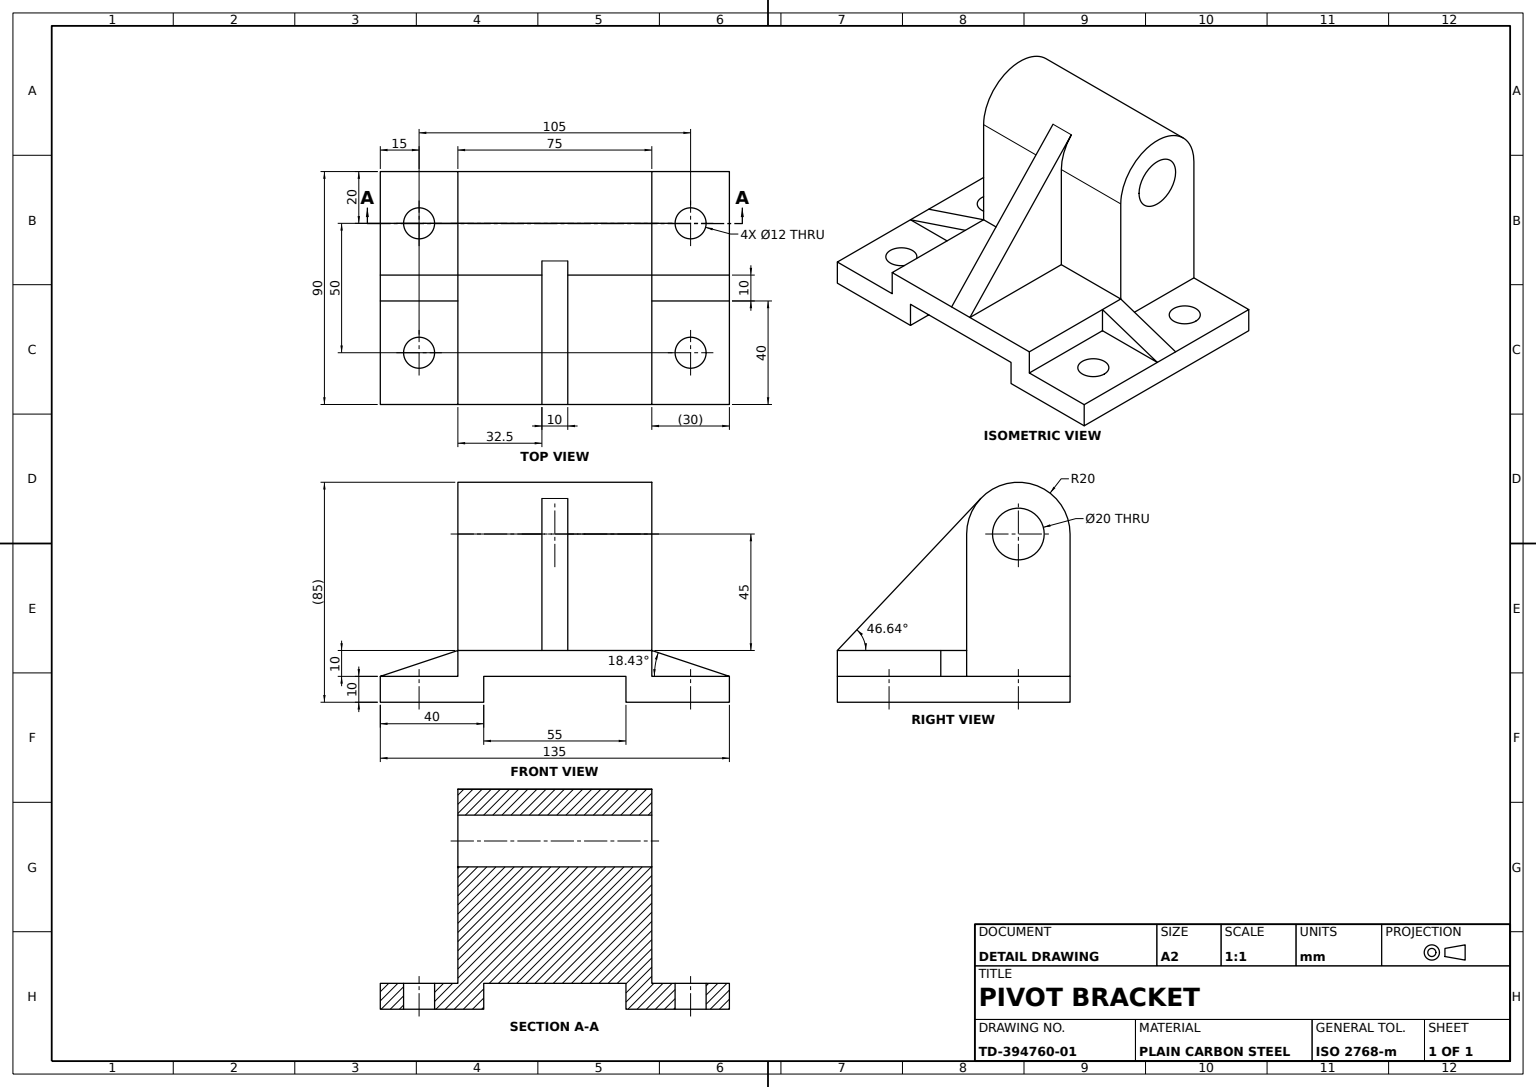
SolidWorks part; units mm, degrees
material "Plain Carbon Steel"
ref_plane "Front Plane" through (0, 0, 0) normal (0, 0, 1) x (1, 0, 0)
ref_plane "Top Plane" through (0, 0, 0) normal (0, 1, 0) x (1, 0, 0)
ref_plane "Right Plane" through (0, 0, 0) normal (1, 0, 0) x (0, 0, -1)
sketch "Base Plate Profile" plane through (0, 0, 0) normal (0, 0, 1) x (1, 0, 0)
  line L0 (-67.5, 0) -> (-27.5, 0)
  line L1 (-27.5, 0) -> (-27.5, 10)
  line L2 (-27.5, 10) -> (27.5, 10)
  line L3 (27.5, 10) -> (27.5, 0)
  line L4 (27.5, 0) -> (67.5, 0)
  line L5 (67.5, 0) -> (67.5, 10)
  line L7 (-67.5, 10) -> (-67.5, 0)
  line L8 (67.5, 10) -> (37.5, 10)
  line L9 (37.5, 10) -> (37.5, 20)
  line L10 (37.5, 20) -> (-37.5, 20)
  line L11 (-37.5, 20) -> (-37.5, 10)
  line L12 (-37.5, 10) -> (-67.5, 10)
  line L13 (0, 0) -> (0, 63.9926) construction
  line L14 (0, 0) -> (111.5972, 0) construction
  dimension "D1" = 55
  dimension "D2" = 135
  dimension "D3" = 75
  dimension "D4" = 10
  dimension "D5" = 10
  dimension "D6" = 10
  dimension "D7" = 10
extrude "Base Plate" add sketch "Base Plate Profile" along normal mid plane 90 contours L2 L3 L4 L5 L8 L9 L10 L11 L12 L7 L0 L1
sketch "Mounting Holes Sketch" plane through (0, 10, 0) normal (0, 1, 0) x (1, 0, 0)
  line L0 (0, 0) -> (0, -31.826) construction
  line L1 (67.5, -45) -> (37.5, -45) construction
  line L2 (67.5, 45) -> (37.5, 45) construction
  line L3 (37.5, -45) -> (37.5, 45) construction
  line L4 (37.5, -45) -> (37.5, 45) construction
  circle A0 centre (52.5, -25) radius 6
  circle A1 centre (52.5, 25) radius 6
  circle A2 centre (-52.5, 25) radius 6
  circle A3 centre (-52.5, -25) radius 6
  dimension "D1" = 12
  dimension "D2" = 12
  dimension "D3" = 20
  dimension "D4" = 20
  dimension "D5" = 15
  dimension "D6" = 15
extrude "Mounting Holes" cut sketch "Mounting Holes Sketch" against normal blind 40
sketch "Pivot Boss Profile" plane through (37.5, 0, 0) normal (1, 0, 0) x (0, 0, -1)
  line L0 (45, 20) -> (5, 20)
  line L1 (-45, 20) -> (45, 20) construction
  line L2 (5, 20) -> (5, 65)
  line L3 (45, 65) -> (45, 20)
  arc A0 (5, 65) -> (45, 65) centre (25, 65) cw
  circle A1 centre (25, 65) radius 10
  dimension "D2" = 20
  dimension "D3" = 20
  dimension "D1" = 45
extrude "Pivot Boss" add sketch "Pivot Boss Profile" against normal blind 75
sketch "Center Gusset Sketch" plane through (0, 0, 0) normal (1, 0, 0) x (0, 0, -1)
  line L0 (10.4585, 78.7312) -> (-45, 20)
  line L1 (-45, 10) -> (-45, 20) construction
  line L2 (-45, 20) -> (5, 20) construction
  arc A0 (45, 65) -> (5, 65) centre (25, 65) ccw construction
rib "Center Gusset Rib" sketch "Center Gusset Sketch" sketch "Center Gusset Sketch" thickness 10 extrusion direction parallel to sketch draft on no parameters "D1"=10
sketch "Side Gusset Sketch" plane through (0, 0, 0) normal (0, 0, 1) x (1, 0, 0)
  line L0 (-37.5, 20) -> (-67.5, 10)
rib "Side Gusset Rib" sketch "Side Gusset Sketch" sketch "Side Gusset Sketch" thickness 10 extrusion direction parallel to sketch draft on no parameters "D1"=10
mirror "Side Gusset Mirror" about plane through (0, 0, 0) normal (1, 0, 0) of "Side Gusset Rib"
